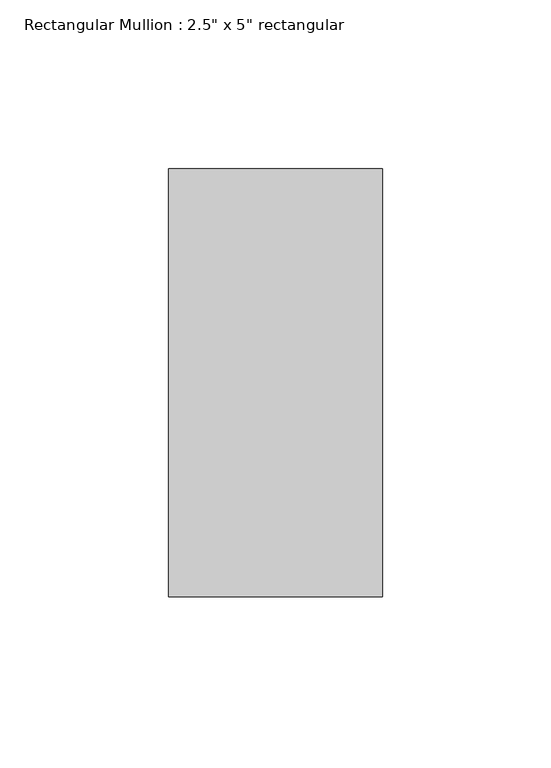
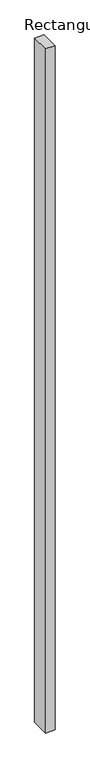
"""IFC4 building model written with IfcOpenShell, lengths in millimetres: member geometry."""

from ifc_helpers import new_model, si_unit, frame, origin, place, context, project, spatial, polyline, outline, extrude, source, transform, mapped, element, save


def member_e63cd10b(model_context):
    return source(origin(), model_context, "Body", "SweptSolid", [
        extrude(outline(polyline([(0.0, 63.5), (0.0, -63.5), (-63.5, -63.5), (-63.5, 63.5), (0.0, 63.5)])), frame((0.0, 0.0, -4857.75), z_axis=(0.0, 0.0, 1.0), x_axis=(1.0, 0.0, 0.0)), (0.0, 0.0, 1.0), 4857.75),
    ])


if __name__ == "__main__":
    model = new_model("IFC4")
    model_context = context("Model", 3, world=origin())
    ifc_project = project(units=[si_unit("LENGTHUNIT", "METRE", prefix="MILLI")], contexts=[model_context])
    site = spatial("IfcSite", under=ifc_project)
    building = spatial("IfcBuilding", under=site)
    placement = place(None, origin())
    member_shape = member_e63cd10b(model_context)
    element("IfcMember", 1, ObjectType="Rectangular Mullion : 2.5\" x 5\" rectangular", at=placement, inside=building, context=model_context, shape_type="MappedRepresentation", body=[
        mapped(member_shape, transform((0.0, 0.0, 0.0), x_axis=(1.0, 0.0, 0.0), y_axis=(0.0, 1.0, 0.0), z_axis=(0.0, 0.0, 1.0))),
    ])
    save(model, "model.ifc")

# Revit data of these elements
# Type "Rectangular Mullion : 2.5\" x 5\" rectangular"
#   built-in parameter 1007304 = 0.416667 (stored number, unit not read)
#   built-in parameter 1007301 = 0.104167 (stored number, unit not read)
#   built-in parameter 1007300 = 0.104167 (stored number, unit not read)
# Element 1 (IfcMember, "Rectangular Mullion : 2.5\" x 5\" rectangular")
#   Materials on its faces: "Aluminum"
# Materials
#   "Aluminum": class "Metal", colour RGB 247 247 247, transparency 0, Description = "Aluminum 6061", Cost = 0
